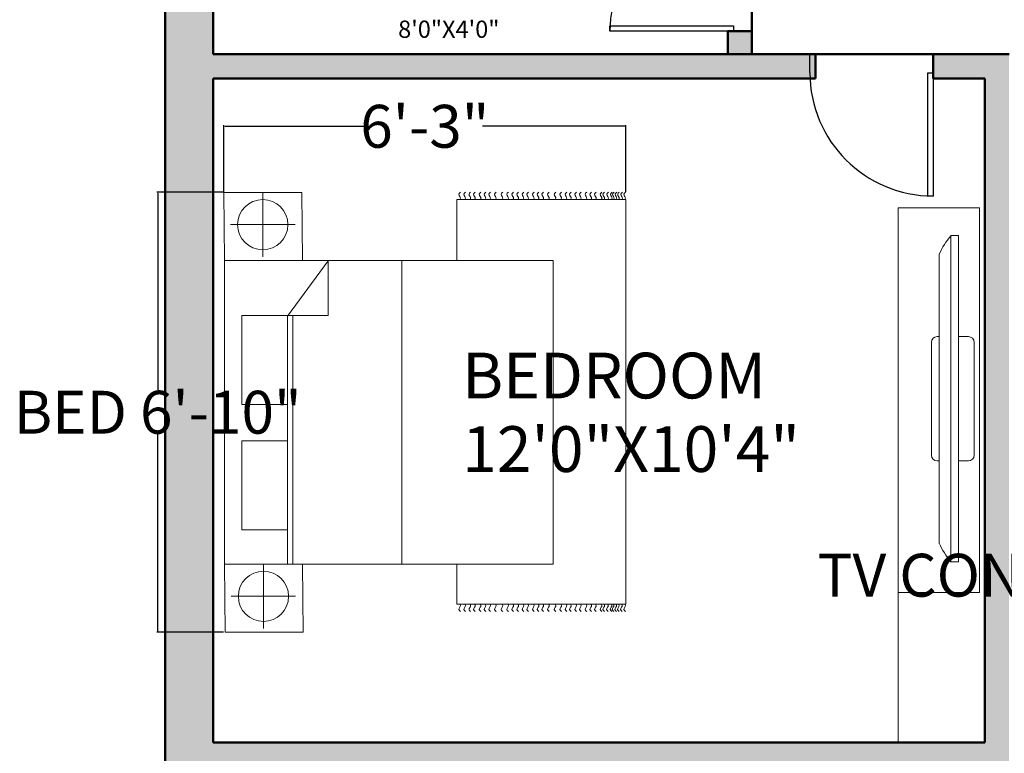
# Model space of a CAD drawing. Units: inches. Extents: x 22042254 to 25404563, y 17568978 to 17626777.
# Tile 37 of 45: x 22179757 to 22179940, y 17626402 to 17626539. Entities that reach past the tile are written whole.
import ezdxf

# ---------------------------------------------------------------- set-up
doc = ezdxf.new("R2010")
doc.units = ezdxf.units.IN
doc.header["$MEASUREMENT"] = 0
for name, color, linetype, lineweight in [('A-ANNO-DIMS', 2, 'Continuous', 18), ('A-AREA-IDEN', 7, 'Continuous', 18), ('A-FURN-PATT', 251, 'Continuous', 13), ('A-WALL-PATT', 244, 'Continuous', 13), ('doors', 4, 'Continuous', 25), ('furniture', 8, 'Continuous', 18), ('walls', 252, 'Continuous', 50)]:
    doc.layers.add(name, color=color, linetype=linetype, lineweight=lineweight)
doc.styles.get("Standard").update_dxf_attribs({"font": 'arial.ttf'})
doc.dimstyles.get("Standard").update_dxf_attribs({"dimtxt": 8, "dimasz": 0.18, "dimexe": 0.18, "dimexo": 0.0625, "dimgap": 0.09, "dimtad": 0, "dimtih": 1, "dimtoh": 1, "dimzin": 0, "dimdsep": 46, "dimlunit": 3, "dimtxsty": 'Standard', "dimcen": 0.09, "dimadec": 0, "dimazin": 0, "dimtfac": 1, "dimtofl": 0, "dimtmove": 0, "dimatfit": 3, "dimfxl": 1, "dimtolj": 1, "dimtzin": 0, "dimarcsym": 0})

# ---------------------------------------------------------------- blocks, each defined once
blk = doc.blocks.new('CARPET')
at = {"layer": 'furniture'}
for p, q in [((-51.53, -98.11), (-51.53, -55.12)), ((-51.53, -55.12), (-41.27, -55.12)), ((36, -55.12), (51.55, -55.12)), ((51.55, -55.12), (51.55, -98.11)), ((51.55, -98.11), (-51.53, -98.11))]:
    blk.add_line(p, q, dxfattribs=at)
for points, knots in [([(-53.37, -55.99), (-53.22, -55.8), (-52.9, -55.41), (-52.34, -55.8), (-51.89, -56.08), (-51.65, -55.91), (-51.53, -55.83)], [0, 0, 0, 0, 0.653278, 1.290138, 1.740457, 2.114451, 2.114451, 2.114451, 2.114451]), ([(-53.37, -57.26), (-53.22, -57.07), (-52.9, -56.67), (-52.34, -57.07), (-51.89, -57.35), (-51.65, -57.17), (-51.53, -57.1)], [0, 0, 0, 0, 0.653278, 1.290138, 1.740457, 2.114451, 2.114451, 2.114451, 2.114451]), ([(53.37, -55.99), (53.22, -55.8), (52.9, -55.41), (52.34, -55.8), (51.89, -56.08), (51.65, -55.91), (51.53, -55.83)], [0, 0, 0, 0, 0.653278, 1.290138, 1.740457, 2.114451, 2.114451, 2.114451, 2.114451]), ([(53.37, -57.26), (53.22, -57.07), (52.9, -56.67), (52.34, -57.07), (51.89, -57.35), (51.65, -57.17), (51.53, -57.1)], [0, 0, 0, 0, 0.653278, 1.290138, 1.740457, 2.114451, 2.114451, 2.114451, 2.114451]), ([(-53.37, -58.59), (-53.22, -58.4), (-52.9, -58.01), (-52.34, -58.4), (-51.89, -58.68), (-51.65, -58.5), (-51.53, -58.43)], [0, 0, 0, 0, 0.653278, 1.290138, 1.740457, 2.114451, 2.114451, 2.114451, 2.114451]), ([(-53.37, -59.78), (-53.22, -59.58), (-52.9, -59.19), (-52.34, -59.58), (-51.89, -59.86), (-51.65, -59.69), (-51.53, -59.61)], [0, 0, 0, 0, 0.653278, 1.290138, 1.740457, 2.114451, 2.114451, 2.114451, 2.114451]), ([(53.37, -58.59), (53.22, -58.4), (52.9, -58.01), (52.34, -58.4), (51.89, -58.68), (51.65, -58.5), (51.53, -58.43)], [0, 0, 0, 0, 0.653278, 1.290138, 1.740457, 2.114451, 2.114451, 2.114451, 2.114451]), ([(53.37, -59.78), (53.22, -59.58), (52.9, -59.19), (52.34, -59.58), (51.89, -59.86), (51.65, -59.69), (51.53, -59.61)], [0, 0, 0, 0, 0.653278, 1.290138, 1.740457, 2.114451, 2.114451, 2.114451, 2.114451]), ([(-53.37, -61.22), (-53.22, -61.02), (-52.9, -60.63), (-52.34, -61.02), (-51.89, -61.3), (-51.65, -61.13), (-51.53, -61.05)], [0, 0, 0, 0, 0.653278, 1.290138, 1.740457, 2.114451, 2.114451, 2.114451, 2.114451]), ([(-53.37, -62.44), (-53.22, -62.25), (-52.9, -61.86), (-52.34, -62.25), (-51.89, -62.53), (-51.65, -62.36), (-51.53, -62.28)], [0, 0, 0, 0, 0.653278, 1.290138, 1.740457, 2.114451, 2.114451, 2.114451, 2.114451]), ([(53.37, -61.22), (53.22, -61.02), (52.9, -60.63), (52.34, -61.02), (51.89, -61.3), (51.65, -61.13), (51.53, -61.05)], [0, 0, 0, 0, 0.653278, 1.290138, 1.740457, 2.114451, 2.114451, 2.114451, 2.114451]), ([(53.37, -62.44), (53.22, -62.25), (52.9, -61.86), (52.34, -62.25), (51.89, -62.53), (51.65, -62.36), (51.53, -62.28)], [0, 0, 0, 0, 0.653278, 1.290138, 1.740457, 2.114451, 2.114451, 2.114451, 2.114451]), ([(-53.37, -63.63), (-53.22, -63.43), (-52.9, -63.04), (-52.34, -63.43), (-51.89, -63.72), (-51.65, -63.54), (-51.53, -63.46)], [0, 0, 0, 0, 0.653278, 1.290138, 1.740457, 2.114451, 2.114451, 2.114451, 2.114451]), ([(-53.37, -65.07), (-53.22, -64.87), (-52.9, -64.48), (-52.34, -64.87), (-51.89, -65.15), (-51.65, -64.98), (-51.53, -64.9)], [0, 0, 0, 0, 0.653278, 1.290138, 1.740457, 2.114451, 2.114451, 2.114451, 2.114451]), ([(53.37, -63.63), (53.22, -63.43), (52.9, -63.04), (52.34, -63.43), (51.89, -63.72), (51.65, -63.54), (51.53, -63.46)], [0, 0, 0, 0, 0.653278, 1.290138, 1.740457, 2.114451, 2.114451, 2.114451, 2.114451]), ([(53.37, -65.07), (53.22, -64.87), (52.9, -64.48), (52.34, -64.87), (51.89, -65.15), (51.65, -64.98), (51.53, -64.9)], [0, 0, 0, 0, 0.653278, 1.290138, 1.740457, 2.114451, 2.114451, 2.114451, 2.114451]), ([(-53.37, -66.76), (-53.22, -66.56), (-52.9, -66.17), (-52.34, -66.56), (-51.89, -66.84), (-51.65, -66.67), (-51.53, -66.59)], [0, 0, 0, 0, 0.653278, 1.290138, 1.740457, 2.114451, 2.114451, 2.114451, 2.114451]), ([(53.37, -66.76), (53.22, -66.56), (52.9, -66.17), (52.34, -66.56), (51.89, -66.84), (51.65, -66.67), (51.53, -66.59)], [0, 0, 0, 0, 0.653278, 1.290138, 1.740457, 2.114451, 2.114451, 2.114451, 2.114451]), ([(-53.37, -68.2), (-53.22, -68), (-52.9, -67.61), (-52.34, -68), (-51.89, -68.28), (-51.65, -68.11), (-51.53, -68.03)], [0, 0, 0, 0, 0.653278, 1.290138, 1.740457, 2.114451, 2.114451, 2.114451, 2.114451]), ([(-53.37, -69.53), (-53.22, -69.33), (-52.9, -68.94), (-52.34, -69.33), (-51.89, -69.61), (-51.65, -69.44), (-51.53, -69.36)], [0, 0, 0, 0, 0.653278, 1.290138, 1.740457, 2.114451, 2.114451, 2.114451, 2.114451]), ([(53.37, -68.2), (53.22, -68), (52.9, -67.61), (52.34, -68), (51.89, -68.28), (51.65, -68.11), (51.53, -68.03)], [0, 0, 0, 0, 0.653278, 1.290138, 1.740457, 2.114451, 2.114451, 2.114451, 2.114451]), ([(53.37, -69.53), (53.22, -69.33), (52.9, -68.94), (52.34, -69.33), (51.89, -69.61), (51.65, -69.44), (51.53, -69.36)], [0, 0, 0, 0, 0.653278, 1.290138, 1.740457, 2.114451, 2.114451, 2.114451, 2.114451]), ([(-53.37, -70.79), (-53.22, -70.6), (-52.9, -70.21), (-52.34, -70.6), (-51.89, -70.88), (-51.65, -70.7), (-51.53, -70.63)], [0, 0, 0, 0, 0.653278, 1.290138, 1.740457, 2.114451, 2.114451, 2.114451, 2.114451]), ([(-53.37, -72.12), (-53.22, -71.93), (-52.9, -71.54), (-52.34, -71.93), (-51.89, -72.21), (-51.65, -72.04), (-51.53, -71.96)], [0, 0, 0, 0, 0.653278, 1.290138, 1.740457, 2.114451, 2.114451, 2.114451, 2.114451]), ([(53.37, -70.79), (53.22, -70.6), (52.9, -70.21), (52.34, -70.6), (51.89, -70.88), (51.65, -70.7), (51.53, -70.63)], [0, 0, 0, 0, 0.653278, 1.290138, 1.740457, 2.114451, 2.114451, 2.114451, 2.114451]), ([(53.37, -72.12), (53.22, -71.93), (52.9, -71.54), (52.34, -71.93), (51.89, -72.21), (51.65, -72.04), (51.53, -71.96)], [0, 0, 0, 0, 0.653278, 1.290138, 1.740457, 2.114451, 2.114451, 2.114451, 2.114451]), ([(-53.37, -73.31), (-53.22, -73.11), (-52.9, -72.72), (-52.34, -73.11), (-51.89, -73.4), (-51.65, -73.22), (-51.53, -73.14)], [0, 0, 0, 0, 0.653278, 1.290138, 1.740457, 2.114451, 2.114451, 2.114451, 2.114451]), ([(-53.37, -74.75), (-53.22, -74.55), (-52.9, -74.16), (-52.34, -74.55), (-51.89, -74.83), (-51.65, -74.66), (-51.53, -74.58)], [0, 0, 0, 0, 0.653278, 1.290138, 1.740457, 2.114451, 2.114451, 2.114451, 2.114451]), ([(53.37, -73.31), (53.22, -73.11), (52.9, -72.72), (52.34, -73.11), (51.89, -73.4), (51.65, -73.22), (51.53, -73.14)], [0, 0, 0, 0, 0.653278, 1.290138, 1.740457, 2.114451, 2.114451, 2.114451, 2.114451]), ([(53.37, -74.75), (53.22, -74.55), (52.9, -74.16), (52.34, -74.55), (51.89, -74.83), (51.65, -74.66), (51.53, -74.58)], [0, 0, 0, 0, 0.653278, 1.290138, 1.740457, 2.114451, 2.114451, 2.114451, 2.114451]), ([(-53.37, -75.98), (-53.22, -75.78), (-52.9, -75.39), (-52.34, -75.78), (-51.89, -76.06), (-51.65, -75.89), (-51.53, -75.81)], [0, 0, 0, 0, 0.653278, 1.290138, 1.740457, 2.114451, 2.114451, 2.114451, 2.114451]), ([(-53.37, -77.16), (-53.22, -76.96), (-52.9, -76.57), (-52.34, -76.96), (-51.89, -77.25), (-51.65, -77.07), (-51.53, -76.99)], [0, 0, 0, 0, 0.653278, 1.290138, 1.740457, 2.114451, 2.114451, 2.114451, 2.114451]), ([(53.37, -75.98), (53.22, -75.78), (52.9, -75.39), (52.34, -75.78), (51.89, -76.06), (51.65, -75.89), (51.53, -75.81)], [0, 0, 0, 0, 0.653278, 1.290138, 1.740457, 2.114451, 2.114451, 2.114451, 2.114451]), ([(53.37, -77.16), (53.22, -76.96), (52.9, -76.57), (52.34, -76.96), (51.89, -77.25), (51.65, -77.07), (51.53, -76.99)], [0, 0, 0, 0, 0.653278, 1.290138, 1.740457, 2.114451, 2.114451, 2.114451, 2.114451]), ([(-53.37, -78.6), (-53.22, -78.4), (-52.9, -78.01), (-52.34, -78.4), (-51.89, -78.68), (-51.65, -78.51), (-51.53, -78.43)], [0, 0, 0, 0, 0.653278, 1.290138, 1.740457, 2.114451, 2.114451, 2.114451, 2.114451]), ([(-53.37, -80.29), (-53.22, -80.09), (-52.9, -79.7), (-52.34, -80.09), (-51.89, -80.37), (-51.65, -80.2), (-51.53, -80.12)], [0, 0, 0, 0, 0.653278, 1.290138, 1.740457, 2.114451, 2.114451, 2.114451, 2.114451]), ([(53.37, -78.6), (53.22, -78.4), (52.9, -78.01), (52.34, -78.4), (51.89, -78.68), (51.65, -78.51), (51.53, -78.43)], [0, 0, 0, 0, 0.653278, 1.290138, 1.740457, 2.114451, 2.114451, 2.114451, 2.114451]), ([(53.37, -80.29), (53.22, -80.09), (52.9, -79.7), (52.34, -80.09), (51.89, -80.37), (51.65, -80.2), (51.53, -80.12)], [0, 0, 0, 0, 0.653278, 1.290138, 1.740457, 2.114451, 2.114451, 2.114451, 2.114451]), ([(-53.37, -81.73), (-53.22, -81.53), (-52.9, -81.14), (-52.34, -81.53), (-51.89, -81.81), (-51.65, -81.64), (-51.53, -81.56)], [0, 0, 0, 0, 0.653278, 1.290138, 1.740457, 2.114451, 2.114451, 2.114451, 2.114451]), ([(-53.37, -83.06), (-53.22, -82.86), (-52.9, -82.47), (-52.34, -82.86), (-51.89, -83.14), (-51.65, -82.97), (-51.53, -82.89)], [0, 0, 0, 0, 0.653278, 1.290138, 1.740457, 2.114451, 2.114451, 2.114451, 2.114451]), ([(53.37, -81.73), (53.22, -81.53), (52.9, -81.14), (52.34, -81.53), (51.89, -81.81), (51.65, -81.64), (51.53, -81.56)], [0, 0, 0, 0, 0.653278, 1.290138, 1.740457, 2.114451, 2.114451, 2.114451, 2.114451]), ([(53.37, -83.06), (53.22, -82.86), (52.9, -82.47), (52.34, -82.86), (51.89, -83.14), (51.65, -82.97), (51.53, -82.89)], [0, 0, 0, 0, 0.653278, 1.290138, 1.740457, 2.114451, 2.114451, 2.114451, 2.114451]), ([(-53.37, -84.18), (-53.22, -83.99), (-52.9, -83.6), (-52.34, -83.99), (-51.89, -84.27), (-51.65, -84.09), (-51.53, -84.02)], [0, 0, 0, 0, 0.653278, 1.290138, 1.740457, 2.114451, 2.114451, 2.114451, 2.114451]), ([(-53.37, -85.51), (-53.22, -85.32), (-52.9, -84.93), (-52.34, -85.32), (-51.89, -85.6), (-51.65, -85.42), (-51.53, -85.35)], [0, 0, 0, 0, 0.653278, 1.290138, 1.740457, 2.114451, 2.114451, 2.114451, 2.114451]), ([(53.37, -84.18), (53.22, -83.99), (52.9, -83.6), (52.34, -83.99), (51.89, -84.27), (51.65, -84.09), (51.53, -84.02)], [0, 0, 0, 0, 0.653278, 1.290138, 1.740457, 2.114451, 2.114451, 2.114451, 2.114451]), ([(53.37, -85.51), (53.22, -85.32), (52.9, -84.93), (52.34, -85.32), (51.89, -85.6), (51.65, -85.42), (51.53, -85.35)], [0, 0, 0, 0, 0.653278, 1.290138, 1.740457, 2.114451, 2.114451, 2.114451, 2.114451]), ([(-53.37, -86.7), (-53.22, -86.5), (-52.9, -86.11), (-52.34, -86.5), (-51.89, -86.78), (-51.65, -86.61), (-51.53, -86.53)], [0, 0, 0, 0, 0.653278, 1.290138, 1.740457, 2.114451, 2.114451, 2.114451, 2.114451]), ([(-53.37, -88.14), (-53.22, -87.94), (-52.9, -87.55), (-52.34, -87.94), (-51.89, -88.22), (-51.65, -88.05), (-51.53, -87.97)], [0, 0, 0, 0, 0.653278, 1.290138, 1.740457, 2.114451, 2.114451, 2.114451, 2.114451]), ([(53.37, -86.7), (53.22, -86.5), (52.9, -86.11), (52.34, -86.5), (51.89, -86.78), (51.65, -86.61), (51.53, -86.53)], [0, 0, 0, 0, 0.653278, 1.290138, 1.740457, 2.114451, 2.114451, 2.114451, 2.114451]), ([(53.37, -88.14), (53.22, -87.94), (52.9, -87.55), (52.34, -87.94), (51.89, -88.22), (51.65, -88.05), (51.53, -87.97)], [0, 0, 0, 0, 0.653278, 1.290138, 1.740457, 2.114451, 2.114451, 2.114451, 2.114451]), ([(-53.37, -89.36), (-53.22, -89.17), (-52.9, -88.78), (-52.34, -89.17), (-51.89, -89.45), (-51.65, -89.28), (-51.53, -89.2)], [0, 0, 0, 0, 0.653278, 1.290138, 1.740457, 2.114451, 2.114451, 2.114451, 2.114451]), ([(-53.37, -90.55), (-53.22, -90.35), (-52.9, -89.96), (-52.34, -90.35), (-51.89, -90.64), (-51.65, -90.46), (-51.53, -90.38)], [0, 0, 0, 0, 0.653278, 1.290138, 1.740457, 2.114451, 2.114451, 2.114451, 2.114451]), ([(53.37, -89.36), (53.22, -89.17), (52.9, -88.78), (52.34, -89.17), (51.89, -89.45), (51.65, -89.28), (51.53, -89.2)], [0, 0, 0, 0, 0.653278, 1.290138, 1.740457, 2.114451, 2.114451, 2.114451, 2.114451]), ([(53.37, -90.55), (53.22, -90.35), (52.9, -89.96), (52.34, -90.35), (51.9, -90.63), (51.66, -90.47), (51.55, -90.4)], [0, 0, 0, 0, 0.653278, 1.290138, 1.740457, 2.0926, 2.0926, 2.0926, 2.0926]), ([(-53.37, -91.99), (-53.22, -91.79), (-52.9, -91.4), (-52.34, -91.79), (-51.89, -92.07), (-51.65, -91.9), (-51.53, -91.82)], [0, 0, 0, 0, 0.653278, 1.290138, 1.740457, 2.114451, 2.114451, 2.114451, 2.114451]), ([(-53.37, -92.69), (-53.22, -92.48), (-52.9, -92.08), (-52.35, -92.49), (-51.89, -92.77), (-51.65, -92.6), (-51.53, -92.52)], [0, 0, 0, 0, 0.663904, 1.307406, 1.757725, 2.131719, 2.131719, 2.131719, 2.131719]), ([(53.37, -91.99), (53.22, -91.79), (52.9, -91.4), (52.34, -91.79), (51.9, -92.07), (51.66, -91.91), (51.55, -91.83)], [0, 0, 0, 0, 0.653278, 1.290138, 1.740457, 2.0926, 2.0926, 2.0926, 2.0926]), ([(53.37, -92.69), (53.22, -92.49), (52.9, -92.09), (52.34, -92.49), (51.9, -92.77), (51.66, -92.61), (51.55, -92.53)], [0, 0, 0, 0, 0.656792, 1.295826, 1.746145, 2.098292, 2.098292, 2.098292, 2.098292]), ([(-53.37, -93.61), (-53.22, -93.42), (-52.9, -93.03), (-52.34, -93.42), (-51.89, -93.7), (-51.65, -93.52), (-51.53, -93.45)], [0, 0, 0, 0, 0.653278, 1.290138, 1.740457, 2.114451, 2.114451, 2.114451, 2.114451]), ([(-53.37, -94.55), (-53.22, -94.35), (-52.9, -93.96), (-52.34, -94.35), (-51.89, -94.63), (-51.65, -94.46), (-51.53, -94.38)], [0, 0, 0, 0, 0.653278, 1.290138, 1.740457, 2.114451, 2.114451, 2.114451, 2.114451]), ([(-53.37, -95.05), (-53.22, -94.85), (-52.9, -94.46), (-52.34, -94.85), (-51.89, -95.14), (-51.65, -94.96), (-51.53, -94.88)], [0, 0, 0, 0, 0.653278, 1.290138, 1.740457, 2.114451, 2.114451, 2.114451, 2.114451]), ([(53.37, -93.66), (53.22, -93.46), (52.9, -93.07), (52.34, -93.46), (51.9, -93.74), (51.66, -93.58), (51.55, -93.5)], [0, 0, 0, 0, 0.653278, 1.290138, 1.740457, 2.0926, 2.0926, 2.0926, 2.0926]), ([(53.37, -94.59), (53.22, -94.4), (52.9, -94.01), (52.34, -94.4), (51.9, -94.68), (51.66, -94.51), (51.55, -94.44)], [0, 0, 0, 0, 0.653278, 1.290138, 1.740457, 2.0926, 2.0926, 2.0926, 2.0926]), ([(53.37, -95.1), (53.22, -94.9), (52.9, -94.51), (52.34, -94.9), (51.9, -95.18), (51.66, -95.02), (51.55, -94.94)], [0, 0, 0, 0, 0.653278, 1.290138, 1.740457, 2.0926, 2.0926, 2.0926, 2.0926]), ([(-53.37, -95.73), (-53.22, -95.54), (-52.9, -95.15), (-52.34, -95.54), (-51.89, -95.82), (-51.65, -95.65), (-51.53, -95.57)], [0, 0, 0, 0, 0.653278, 1.290138, 1.740457, 2.114451, 2.114451, 2.114451, 2.114451]), ([(-53.37, -96.38), (-53.22, -96.18), (-52.9, -95.79), (-52.34, -96.18), (-51.89, -96.47), (-51.65, -96.29), (-51.53, -96.21)], [0, 0, 0, 0, 0.653278, 1.290138, 1.740457, 2.114451, 2.114451, 2.114451, 2.114451]), ([(-53.37, -97.17), (-53.22, -96.98), (-52.9, -96.59), (-52.34, -96.98), (-51.89, -97.26), (-51.65, -97.08), (-51.53, -97.01)], [0, 0, 0, 0, 0.653278, 1.290138, 1.740457, 2.114451, 2.114451, 2.114451, 2.114451]), ([(-53.37, -97.99), (-53.22, -97.79), (-52.9, -97.4), (-52.34, -97.79), (-51.89, -98.08), (-51.65, -97.9), (-51.53, -97.82)], [0, 0, 0, 0, 0.653278, 1.290138, 1.740457, 2.114451, 2.114451, 2.114451, 2.114451]), ([(53.37, -95.78), (53.22, -95.58), (52.9, -95.19), (52.34, -95.58), (51.89, -95.86), (51.65, -95.69), (51.53, -95.61)], [0, 0, 0, 0, 0.653278, 1.290138, 1.740457, 2.114451, 2.114451, 2.114451, 2.114451]), ([(53.37, -96.43), (53.22, -96.23), (52.9, -95.84), (52.34, -96.23), (51.89, -96.51), (51.65, -96.34), (51.53, -96.26)], [0, 0, 0, 0, 0.653278, 1.290138, 1.740457, 2.114451, 2.114451, 2.114451, 2.114451]), ([(53.37, -97.22), (53.22, -97.02), (52.9, -96.63), (52.34, -97.02), (51.89, -97.3), (51.65, -97.13), (51.53, -97.05)], [0, 0, 0, 0, 0.653278, 1.290138, 1.740457, 2.114451, 2.114451, 2.114451, 2.114451]), ([(53.37, -97.99), (53.22, -97.79), (52.9, -97.4), (52.34, -97.79), (51.89, -98.08), (51.65, -97.9), (51.53, -97.82)], [0, 0, 0, 0, 0.653278, 1.290138, 1.740457, 2.114451, 2.114451, 2.114451, 2.114451])]:
    blk.add_open_spline(points, degree=3, knots=knots, dxfattribs=at)
blk = doc.blocks.new('A$C58D270C6')
at = {"layer": 'furniture'}
for p, q in [((9.09, 124.13), (9.09, 108.87)), ((1.46, 116.5), (16.73, 116.5)), ((14.97, 94.84), (24.62, 107.92)), ((24.62, 94.93), (24.62, 107.92)), ((42.08, 108), (42.08, 36)), ((14.97, 94.93), (24.62, 94.93)), ((14.97, 94.84), (14.97, 36)), ((16.22, 94.93), (16.22, 36)), ((9.25, 36), (9.25, 20.74)), ((1.62, 28.37), (16.88, 28.37))]:
    blk.add_line(p, q, dxfattribs=at)
for points in [[(18.5, 108), (18.34, 124.13), (-0.16, 124.13), (0, 108)], [(0, 108), (77.91, 108), (77.91, 36), (0, 36)], [(4.09, 94.93), (14.97, 94.93), (14.97, 73.83), (4.09, 73.83)], [(4.09, 65.23), (14.97, 65.23), (14.97, 44.13), (4.09, 44.13)], [(18.65, 19.87), (18.5, 36), (0, 36), (0.16, 19.87)]]:
    blk.add_lwpolyline(points, close=True, dxfattribs=at)
for centre in [(9.09, 116.5), (9.25, 28.37)]:
    blk.add_circle(centre, 5.95, dxfattribs=at)
at = {"layer": 'furniture', "xscale": 0.9312884925094044, "yscale": 0.9312884925094044, "zscale": 0.9312884925094044, "rotation": 90}
blk.add_blockref('CARPET', (3.79, 74.47), dxfattribs=at)
blk = doc.blocks.new('*U24')
for p, q in [((0, 0), (0, -6)), ((40, 0), (40, -6))]:
    blk.add_line(p, q)
blk.add_lwpolyline([(0, 0), (0, 40), (1.75, 40), (1.75, 0)], close=True)
blk.add_arc((0, 0), 40, 0, 90)
blk = doc.blocks.new('PLASMA-LARGE')
at = {"layer": 'furniture'}
for p, q in [((-7.26, 0), (7.26, 0)), ((-18.61, -1), (18.61, -1)), ((-8, -1), (-8, -0.74)), ((8, -1), (8, -0.74)), ((-21, -2.5), (21, -2.5)), ((-21, -2.5), (-21, -3.5)), ((21, -2.5), (21, -3.5)), ((-21, -3.5), (21, -3.5)), ((-8, -3.5), (-8, -4.76)), ((8, -3.5), (8, -4.76)), ((-7.26, -5.5), (7.26, -5.5))]:
    blk.add_line(p, q, dxfattribs=at)
for centre, radius, start, end in [((-7.26, -0.74), 0.744, 90, 180), ((7.26, -0.74), 0.744, 0, 90), ((-13.97, -11.05), 11.07, 114.7602, 129.4175), ((13.97, -11.05), 11.07, 50.5825, 65.2398), ((-7.26, -4.76), 0.744, 180, 270), ((7.26, -4.76), 0.744, 270, 0)]:
    blk.add_arc(centre, radius, start, end, dxfattribs=at)
blk = doc.blocks.new('TV-CONSOLE')
for p, q in [((8.99, 35.63), (-6.22, 35.63)), ((-6.22, 35.63), (-6.22, -36.14)), ((8.99, -36.14), (8.99, 35.63)), ((-6.22, -36.14), (8.99, -36.14))]:
    blk.add_line(p, q)
at = {"xscale": 1.450199298177205, "yscale": 1.450199298177205, "zscale": 1.450199298177205, "rotation": 90}
blk.add_blockref('PLASMA-LARGE', (0, 0), dxfattribs=at)
blk = doc.blocks.new('*D32')
at = {"layer": 'A-ANNO-DIMS', "color": 0, "lineweight": -2, "transparency": 16777216}
for p, q in [((22179794.63, 17626506.52), (22179782.2, 17626506.52)), ((22179782.38, 17626506.34), (22179782.38, 17626469.63)), ((22179782.38, 17626424.58), (22179782.38, 17626461.28)), ((22179794.63, 17626424.4), (22179782.2, 17626424.4))]:
    blk.add_line(p, q, dxfattribs=at)
at = {"layer": 'A-ANNO-DIMS', "color": 0, "transparency": 16777216}
for points in [[(22179782.35, 17626506.34), (22179782.41, 17626506.34), (22179782.38, 17626506.52)], [(22179782.35, 17626424.58), (22179782.41, 17626424.58), (22179782.38, 17626424.4)]]:
    blk.add_solid(points, dxfattribs=at)
at = {"layer": 'Defpoints', "color": 0, "transparency": 16777216}
for p in [(22179782.38, 17626506.52), (22179794.7, 17626506.52), (22179794.7, 17626424.4)]:
    blk.add_point(p, dxfattribs=at)
at = {"layer": 'A-ANNO-DIMS', "color": 0, "transparency": 16777216, "insert": (22179782.38, 17626465.46), "char_height": 8, "attachment_point": 5}
blk.add_mtext('\\A1;BED 6\'-10"', dxfattribs=at)
blk = doc.blocks.new('*D33')
at = {"layer": 'A-ANNO-DIMS', "color": 0, "lineweight": -2, "transparency": 16777216}
for p, q in [((22179794.7, 17626506.58), (22179794.7, 17626519.02)), ((22179794.88, 17626518.84), (22179821.47, 17626518.84)), ((22179869.56, 17626518.84), (22179842.96, 17626518.84)), ((22179869.74, 17626506.58), (22179869.74, 17626519.02))]:
    blk.add_line(p, q, dxfattribs=at)
at = {"layer": 'A-ANNO-DIMS', "color": 0, "transparency": 16777216}
for points in [[(22179794.88, 17626518.87), (22179794.88, 17626518.81), (22179794.7, 17626518.84)], [(22179869.56, 17626518.87), (22179869.56, 17626518.81), (22179869.74, 17626518.84)]]:
    blk.add_solid(points, dxfattribs=at)
at = {"layer": 'Defpoints', "color": 0, "transparency": 16777216}
for p in [(22179869.74, 17626518.84), (22179794.7, 17626506.52), (22179869.74, 17626506.52)]:
    blk.add_point(p, dxfattribs=at)
at = {"layer": 'A-ANNO-DIMS', "color": 0, "transparency": 16777216, "insert": (22179832.22, 17626518.84), "char_height": 8, "attachment_point": 5}
blk.add_mtext('\\A1;6\'-3"', dxfattribs=at)
blk = doc.blocks.new('*D40')
at = {"layer": 'A-ANNO-DIMS', "color": 0, "lineweight": -2, "transparency": 16777216}
for p, q in [((22179954.93, 17626464.83), (22179963.98, 17626464.83)), ((22179963.8, 17626464.65), (22179963.8, 17626439.26)), ((22179963.8, 17626405.42), (22179963.8, 17626430.8)), ((22179954.93, 17626405.24), (22179963.98, 17626405.24))]:
    blk.add_line(p, q, dxfattribs=at)
at = {"layer": 'A-ANNO-DIMS', "color": 0, "transparency": 16777216}
for points in [[(22179963.77, 17626464.65), (22179963.83, 17626464.65), (22179963.8, 17626464.83)], [(22179963.77, 17626405.42), (22179963.83, 17626405.42), (22179963.8, 17626405.24)]]:
    blk.add_solid(points, dxfattribs=at)
at = {"layer": 'Defpoints', "color": 0, "transparency": 16777216}
for p in [(22179954.87, 17626464.83), (22179963.8, 17626464.83), (22179954.87, 17626405.24)]:
    blk.add_point(p, dxfattribs=at)
at = {"layer": 'A-ANNO-DIMS', "color": 0, "transparency": 16777216, "insert": (22179963.8, 17626435.03), "char_height": 8, "attachment_point": 5}
blk.add_mtext('\\A1;TV CONSOLE 4\'-11 1/2"', dxfattribs=at)

msp = doc.modelspace()

# ---------------------------------------------------------------- hatches: boundary and pattern name
at = {"layer": 'A-FURN-PATT'}
h = msp.add_hatch(color=256, dxfattribs=at)
h.dxf.hatch_style = 1
h.paths.add_polyline_path([(22179794.695, 17626506.484), (22179809.26, 17626506.484), (22179809.382, 17626493.783), (22179838.221, 17626493.783), (22179838.221, 17626505.187), (22179869.738, 17626505.187), (22179869.738, 17626429.601), (22179838.221, 17626429.601), (22179838.221, 17626437.096), (22179809.382, 17626437.096), (22179809.505, 17626424.396), (22179794.94, 17626424.396), (22179794.818, 17626437.096), (22179794.818, 17626493.783)], flags=0)
h.paths.add_polyline_path([(22179797.289, 17626500.475, -1), (22179806.666, 17626500.475, -1)], flags=0)
h.paths.add_polyline_path([(22179798.041, 17626483.494), (22179806.658, 17626483.494), (22179814.199, 17626493.722), (22179814.199, 17626483.494), (22179806.658, 17626483.494), (22179806.607, 17626483.426), (22179806.607, 17626443.497), (22179798.041, 17626443.497), (22179798.041, 17626460.107), (22179806.607, 17626460.107), (22179806.607, 17626466.884), (22179798.041, 17626466.884)], flags=0)
h.paths.add_polyline_path([(22179806.789, 17626431.088, -1), (22179797.412, 17626431.088, -1)], flags=0)
h.paths.add_polyline_path([(22179920.515, 17626503.598), (22179935.729, 17626503.598), (22179935.729, 17626431.832), (22179920.515, 17626431.832)], flags=0)
h.paths.add_polyline_path([(22179928.185, 17626494.952, -0.0640419), (22179930.36, 17626498.421), (22179931.81, 17626498.421), (22179931.81, 17626479.569), (22179933.631, 17626479.569, -0.4142136), (22179934.711, 17626478.489), (22179934.711, 17626457.445, -0.4142136), (22179933.631, 17626456.365), (22179931.81, 17626456.365), (22179931.81, 17626437.513), (22179930.36, 17626437.513, -0.0640419), (22179928.185, 17626440.982), (22179928.185, 17626456.365), (22179927.814, 17626456.365, -0.4142136), (22179926.735, 17626457.445), (22179926.735, 17626478.489, -0.4142136), (22179927.814, 17626479.569), (22179928.185, 17626479.569)], flags=0)
h.paths.add_polyline_path([(22179836.995, 17626451.976), (22179902.189, 17626451.976), (22179902.189, 17626465.064), (22179836.995, 17626465.064)], flags=8)
h.paths.add_polyline_path([(22179836.966, 17626465.674), (22179903.069, 17626465.674), (22179903.069, 17626478.937), (22179836.966, 17626478.937)], flags=8)
at = {"layer": 'A-WALL-PATT'}
h = msp.add_hatch(color=256, dxfattribs=at)
h.dxf.hatch_style = 1
h.paths.add_polyline_path([(22179792.734, 17626580.28), (22179888.734, 17626580.28), (22179888.734, 17626559.623), (22179893.234, 17626559.623), (22179893.234, 17626580.28), (22179900.438, 17626580.28), (22179900.438, 17626584.78), (22179792.734, 17626584.78), (22179792.734, 17626728.78), (22180134.734, 17626728.78), (22180134.734, 17626584.78), (22180035.602, 17626584.78), (22180004.432, 17626584.78), (22180001.734, 17626584.78), (22180001.734, 17626580.28), (22180134.734, 17626580.28), (22180134.734, 17626404.28), (22180064.487, 17626404.28), (22180064.487, 17626399.78), (22180134.734, 17626399.78), (22180134.734, 17626197.78), (22180143.734, 17626197.78), (22180143.734, 17626737.78), (22179783.734, 17626737.78), (22179783.734, 17626197.78), (22179792.734, 17626197.78), (22179792.734, 17626394.78), (22179936.734, 17626394.78), (22179936.734, 17626383.208), (22179941.234, 17626383.208), (22179941.234, 17626532.28), (22179927.066, 17626532.28), (22179927.066, 17626527.78), (22179928.072, 17626527.78), (22179936.734, 17626527.78), (22179936.734, 17626403.78), (22179792.734, 17626403.78), (22179792.734, 17626527.78), (22179905.094, 17626527.78), (22179905.094, 17626532.28), (22179792.734, 17626532.28)])
h = msp.add_hatch(color=256, dxfattribs=at)
h.dxf.hatch_style = 1
h.paths.add_polyline_path([(22179941.234, 17626336.599), (22179936.734, 17626336.599), (22179936.734, 17626270.28), (22180065.734, 17626270.28), (22180065.734, 17626197.78), (22180074.734, 17626197.78), (22180074.734, 17626279.28), (22180025.734, 17626279.28), (22180025.734, 17626404.28), (22180021.234, 17626404.28), (22180021.234, 17626279.28), (22179941.234, 17626279.28), (22179941.234, 17626327.28), (22179991.805, 17626327.28), (22179991.805, 17626331.78), (22179941.234, 17626331.78)])
h.paths.add_polyline_path([(22180036.005, 17626206.78), (22179936.734, 17626206.78), (22179936.734, 17626197.78), (22180036.005, 17626197.78)], flags=17)
h.paths.add_polyline_path([(22179836.995, 17626451.976), (22179902.189, 17626451.976), (22179902.189, 17626465.064), (22179836.995, 17626465.064)], flags=9)
h.paths.add_polyline_path([(22179836.966, 17626465.674), (22179903.069, 17626465.674), (22179903.069, 17626478.937), (22179836.966, 17626478.937)], flags=9)
h.paths.add_polyline_path([(22180055.036, 17626649.533), (22180120.23, 17626649.533), (22180120.23, 17626662.622), (22180055.036, 17626662.622)], flags=9)
h.paths.add_polyline_path([(22180055.007, 17626663.231), (22180121.111, 17626663.231), (22180121.111, 17626676.495), (22180055.007, 17626676.495)], flags=9)
h = msp.add_hatch(color=256, dxfattribs=at)
h.dxf.hatch_style = 1
h.paths.add_polyline_path([(22179893.234, 17626536.599), (22179889.78, 17626536.599), (22179888.734, 17626536.599), (22179888.734, 17626532.28), (22179893.234, 17626532.28)], flags=17)
h.paths.add_polyline_path([(22180021.234, 17626331.78), (22180014.784, 17626331.78), (22180014.784, 17626328.329), (22180014.784, 17626327.28), (22180021.234, 17626327.28)], flags=17)
h.paths.add_polyline_path([(22180079.631, 17626279.28), (22180074.734, 17626279.28), (22180074.734, 17626277.567), (22180079.631, 17626277.567)], flags=17)
h.paths.add_polyline_path([(22179935.729, 17626503.598), (22179935.729, 17626431.832), (22179920.515, 17626431.832), (22179920.515, 17626503.598)], flags=0)
h.paths.add_polyline_path([(22179931.81, 17626498.421), (22179931.81, 17626479.569), (22179933.631, 17626479.569, -0.4142136), (22179934.711, 17626478.489), (22179934.711, 17626457.445, -0.4142136), (22179933.631, 17626456.365), (22179931.81, 17626456.365), (22179931.81, 17626437.513), (22179930.36, 17626437.513, -0.0640419), (22179928.185, 17626440.982), (22179928.185, 17626456.365), (22179927.814, 17626456.365, -0.4142136), (22179926.735, 17626457.445), (22179926.735, 17626478.489, -0.4142136), (22179927.814, 17626479.569), (22179928.185, 17626479.569), (22179928.185, 17626494.952, -0.0640419), (22179930.36, 17626498.421)], flags=0)
h.paths.add_polyline_path([(22179869.738, 17626505.187), (22179869.738, 17626429.601), (22179838.221, 17626429.601), (22179838.221, 17626437.096), (22179809.382, 17626437.096), (22179809.505, 17626424.396), (22179794.94, 17626424.396), (22179794.818, 17626437.096), (22179794.818, 17626493.783), (22179794.695, 17626506.484), (22179809.26, 17626506.484), (22179809.382, 17626493.783), (22179838.221, 17626493.783), (22179838.221, 17626505.187)], flags=0)
h.paths.add_polyline_path([(22179814.199, 17626493.722), (22179814.199, 17626483.494), (22179806.658, 17626483.494), (22179806.607, 17626483.426), (22179806.607, 17626443.497), (22179798.041, 17626443.497), (22179798.041, 17626460.107), (22179806.607, 17626460.107), (22179806.607, 17626466.884), (22179798.041, 17626466.884), (22179798.041, 17626483.494), (22179806.658, 17626483.494)], flags=0)
h.paths.add_polyline_path([(22179806.666, 17626500.475, -1), (22179797.289, 17626500.475, -1)], flags=0)
h.paths.add_polyline_path([(22179806.789, 17626431.088, -1), (22179797.412, 17626431.088, -1)], flags=0)
h.paths.add_polyline_path([(22179836.995, 17626451.976), (22179902.189, 17626451.976), (22179902.189, 17626465.064), (22179836.995, 17626465.064)], flags=8)
h.paths.add_polyline_path([(22179836.966, 17626465.674), (22179903.069, 17626465.674), (22179903.069, 17626478.937), (22179836.966, 17626478.937)], flags=8)

# ---------------------------------------------------------------- linework, layer by layer
at = {"layer": 'furniture'}
msp.add_line((22179920.515, 17626431.832), (22179920.515, 17626403.78), dxfattribs=at)
at = {"layer": 'walls'}
for p, q in [((22179783.734, 17626197.78), (22179783.734, 17626737.78)), ((22179792.734, 17626532.28), (22179792.734, 17626580.28)), ((22179893.234, 17626532.28), (22179893.234, 17626580.28)), ((22179893.234, 17626559.623), (22179893.234, 17626536.599)), ((22179888.734, 17626532.28), (22179888.734, 17626536.599)), ((22179888.734, 17626536.599), (22179893.234, 17626536.599)), ((22179893.234, 17626536.599), (22179888.734, 17626536.599)), ((22179792.734, 17626532.28), (22179941.234, 17626532.28)), ((22179905.094, 17626527.78), (22179905.094, 17626532.28)), ((22179927.066, 17626527.78), (22179927.066, 17626532.28)), ((22179792.734, 17626527.78), (22179905.094, 17626527.78)), ((22179792.734, 17626403.78), (22179792.734, 17626527.78)), ((22179927.066, 17626527.78), (22179928.072, 17626527.78)), ((22179928.072, 17626527.78), (22179936.734, 17626527.78)), ((22179936.734, 17626403.78), (22179936.734, 17626527.78)), ((22179792.734, 17626403.78), (22179936.734, 17626403.78))]:
    msp.add_line(p, q, dxfattribs=at)

# ---------------------------------------------------------------- block references
at = {"layer": 'doors'}
for p, xscale, yscale, zscale, rotation in [((22179889.78, 17626536.599), 0.5755769432943251, 0.5755769432943251, 0.5755769432943251, 90), ((22179927.066, 17626528.829), 0.5750671146789703, 0.5750671146789703, 0.5750671146789703, 180)]:
    msp.add_blockref('*U24', p, dxfattribs=dict(at, xscale=xscale, yscale=yscale, zscale=zscale, rotation=rotation))
at = {"layer": 'furniture', "xscale": 0.7873196543551435, "yscale": 0.7873196543551435, "zscale": 0.7873196543551435}
msp.add_blockref('A$C58D270C6', (22179794.818, 17626408.753), dxfattribs=at)
at = {"layer": 'furniture'}
msp.add_blockref('TV-CONSOLE', (22179926.735, 17626467.967), dxfattribs=at)

# ---------------------------------------------------------------- texts
at = {"layer": 'A-AREA-IDEN'}
for s, height, p in [('8\'0"X4\'0"', 3.2253, (22179827.231, 17626535.349)), ('BEDROOM', 8.5453, (22179839.176, 17626468.03)), ('12\'0"X10\'4"', 8.54529, (22179839.176, 17626454.303))]:
    msp.add_text(s, height=height, dxfattribs=at).set_placement(p)

# ---------------------------------------------------------------- dimensions: what is measured, and where the dimension line sits
at = {"layer": 'A-ANNO-DIMS'}
dim = msp.add_linear_dim(base=(22179869.738, 17626518.841), p1=(22179794.695, 17626506.522), p2=(22179869.738, 17626506.522), dimstyle='Standard', override={"dimdec": 1, "dimlfac": 1, "dimrnd": 0, "dimzin": 1, "dimdsep": 46, "dimlunit": 4, "dimfrac": 2}, dxfattribs=at)
dim.commit()
dim.dimension.update_dxf_attribs({"geometry": '*D33', "text_midpoint": (22179832.217, 17626518.841)})
for base, p1, p2, text, picture, middle in [((22179782.376, 17626506.522), (22179794.695, 17626424.396), (22179794.695, 17626506.522), 'BED <>', '*D32', (22179782.376, 17626465.459)), ((22179963.805, 17626464.828), (22179954.866, 17626405.239), (22179954.866, 17626464.828), 'TV CONSOLE <>', '*D40', (22179963.805, 17626435.034))]:
    dim = msp.add_linear_dim(base=base, p1=p1, p2=p2, angle=90, text=text, dimstyle='Standard', override={"dimdec": 1, "dimlfac": 1, "dimrnd": 0, "dimzin": 1, "dimdsep": 46, "dimlunit": 4, "dimfrac": 2}, dxfattribs=at)
    dim.commit()
    dim.dimension.update_dxf_attribs({"geometry": picture, "text_midpoint": middle})

doc.saveas('drawing.dxf')
